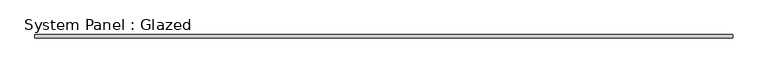
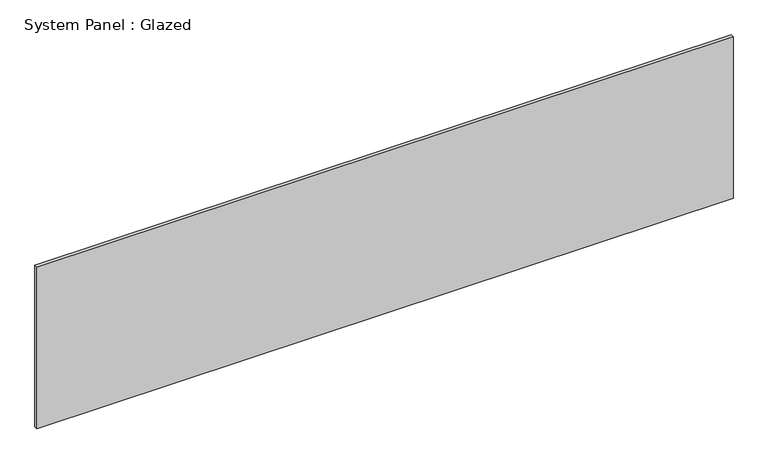
"""IFC4 building model written with IfcOpenShell, lengths in millimetres: plate geometry, System Panel : Glazed."""

from ifc_helpers import new_model, si_unit, origin, origin_with_axes, place, context, project, spatial, polyline, outline, extrude, source, transform, mapped, element, save


def system_panel_glazed_d59597fa(model_context):
    return source(origin(), model_context, "Body", "SweptSolid", [
        extrude(outline(polyline([(2485.6820739, 19.05), (-2485.6820739, 19.05), (-2485.6820739, 44.45), (2485.6820739, 44.45), (2485.6820739, 19.05)])), origin_with_axes(), (0.0, 0.0, 1.0), 1219.2),
    ])


if __name__ == "__main__":
    model = new_model("IFC4")
    model_context = context("Model", 3, world=origin())
    ifc_project = project(units=[si_unit("LENGTHUNIT", "METRE", prefix="MILLI")], contexts=[model_context])
    site = spatial("IfcSite", under=ifc_project)
    building = spatial("IfcBuilding", under=site)
    placement = place(None, origin())
    system_panel_glazed_shape = system_panel_glazed_d59597fa(model_context)
    element("IfcPlate", 1, ObjectType="System Panel : Glazed", at=placement, inside=building, context=model_context, shape_type="MappedRepresentation", body=[
        mapped(system_panel_glazed_shape, transform((0.0, 0.0, 0.0), x_axis=(1.0, 0.0, 0.0), y_axis=(0.0, 1.0, 0.0), z_axis=(0.0, 0.0, 1.0))),
    ])
    save(model, "model.ifc")

# Revit data of these elements
# Type "System Panel : Glazed"
#   Construction Type Id = "GSP4R"
#   Analytic Construction = "1/8 in Pilkington single glazing"
#   Visual Light Transmittance = 0.9
#   Solar Heat Gain Coefficient = 0.86
#   Heat Transfer Coefficient (U) = 1.18115 BTU/(h·ft²·°F)
# Element 1 (IfcPlate, "System Panel : Glazed")
#   Materials on its faces: "Glass"
# Materials
#   "Glass": class "Glass", colour RGB 0 128 192, transparency 0.75, Description = "Soda Lime Glass", Cost = 0
